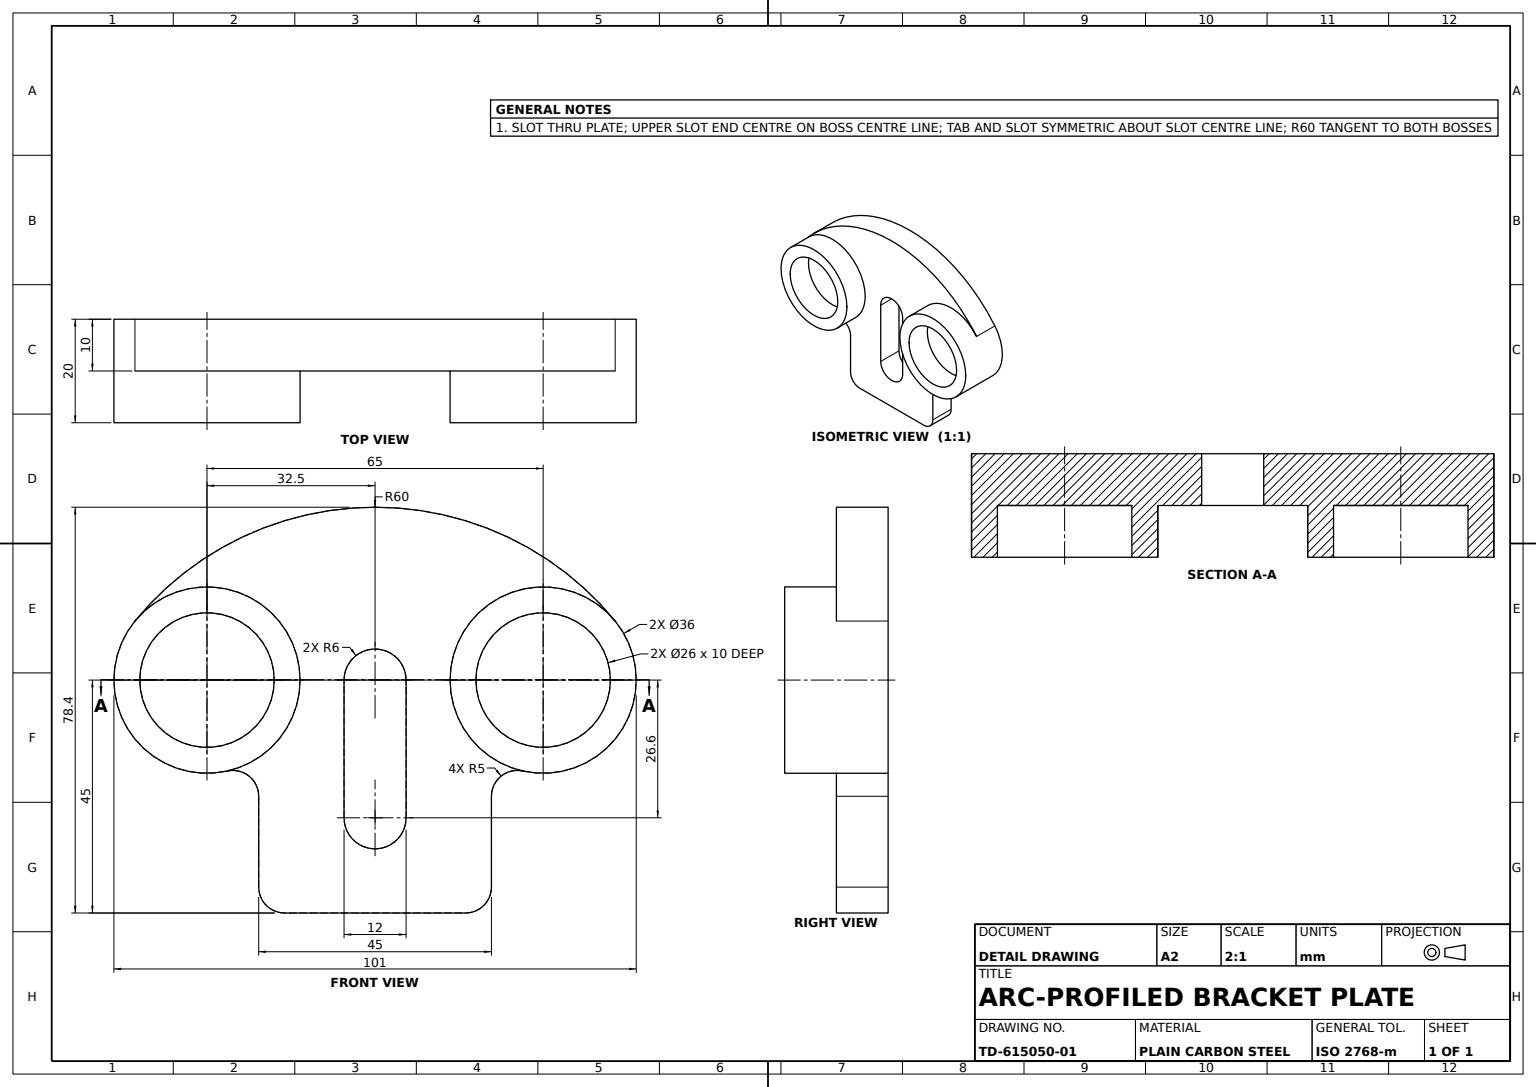
from build123d import *

# Parameters (mm, degrees)
BASE_PLATE_10MM_DEPTH    = 10
BRACKET_PROFILE_SKETCH_R = 13
BASE_PLATE_10MM_2_DEPTH  = 10
BASE_PLATE_10MM_3_DEPTH  = 10
SKETCH1_3_R              = 18
SKETCH1_3_R_2            = 13
HUB_BOSSES_20MM_DEPTH    = 20


with BuildPart() as part:
    # Bracket Profile Sketch → Base Plate 10mm (new body)
    with BuildSketch(Plane.XY):
        with BuildLine():
            ThreePointArc((-22.5, -13.396428811), (-21.035533906, -16.931962717), (-17.5, -18.396428811))
            Line((-17.5, -18.396428811), (17.5, -18.396428811))
            ThreePointArc((17.5, -18.396428811), (21.035533906, -16.931962717), (22.5, -13.396428811))
            Line((22.5, -13.396428811), (22.5, 4.153626868))
            ThreePointArc((22.5, 4.153626868), (24.37228383, 8.054574389), (28.586956623, 9.034049524))
            ThreePointArc((28.586956623, 9.034049524), (17.173285852, 36.042418229), (46.428571429, 38.005101698))
            ThreePointArc((46.428571429, 38.005101698), (0, 60), (-46.428571429, 38.005101698))
            ThreePointArc((-46.428571429, 38.005101698), (-26.446665618, 43.555182996), (-14.5, 26.603571189))
            ThreePointArc((-14.5, 26.603571189), (-18.456589043, 15.34379283), (-28.586956522, 9.034049547))
            ThreePointArc((-28.586956522, 9.034049547), (-24.372283789, 8.054574356), (-22.5, 4.153626868))
            Line((-22.5, 4.153626868), (-22.5, -13.396428811))
        make_face()
        with BuildLine():
            Line((-6, 0), (-6, 26.603571189))
            ThreePointArc((-6, 26.603571189), (0, 32.603571189), (6, 26.603571189))
            Line((6, 26.603571189), (6, 0))
            ThreePointArc((6, 0), (0, -6), (-6, 0))
        make_face(mode=Mode.SUBTRACT)
    extrude(amount=BASE_PLATE_10MM_DEPTH)



with BuildPart() as body_2:
    # Bracket Profile Sketch → Base Plate 10mm 2 (new body)
    with BuildSketch(Plane.XY):
        with Locations((-32.5, 26.603571189)):
            Circle(BRACKET_PROFILE_SKETCH_R)
    extrude(amount=BASE_PLATE_10MM_2_DEPTH)


with BuildPart() as body_3:
    # Bracket Profile Sketch → Base Plate 10mm 3 (new body)
    with BuildSketch(Plane.XY):
        with Locations((32.5, 26.603571189)):
            Circle(BRACKET_PROFILE_SKETCH_R)
    extrude(amount=BASE_PLATE_10MM_3_DEPTH)


with BuildPart() as part_1:
    add(part.part)

    add(body_2.part)  # Hub Bosses 20mm merges body 2

    add(body_3.part)  # Hub Bosses 20mm merges body 3
    # Sketch1_3 → Hub Bosses 20mm (add)
    # profile 1 of 2: a face of its own
    with BuildSketch(Plane.XY):
        with Locations(Location((-32.5, 26.603571189, 0), (0, 0, 140.697224227))):
            Circle(SKETCH1_3_R)
        with Locations((-32.5, 26.603571189)):
            Circle(SKETCH1_3_R_2, mode=Mode.SUBTRACT)
    # profile 2 of 2: a face of its own
    with BuildSketch(Plane.XY):
        with Locations(Location((32.5, 26.603571189, 0), (0, 0, 257.444142201))):
            Circle(SKETCH1_3_R)
        with Locations((32.5, 26.603571189)):
            Circle(SKETCH1_3_R_2, mode=Mode.SUBTRACT)
    extrude(amount=HUB_BOSSES_20MM_DEPTH)


solid = part_1.part
